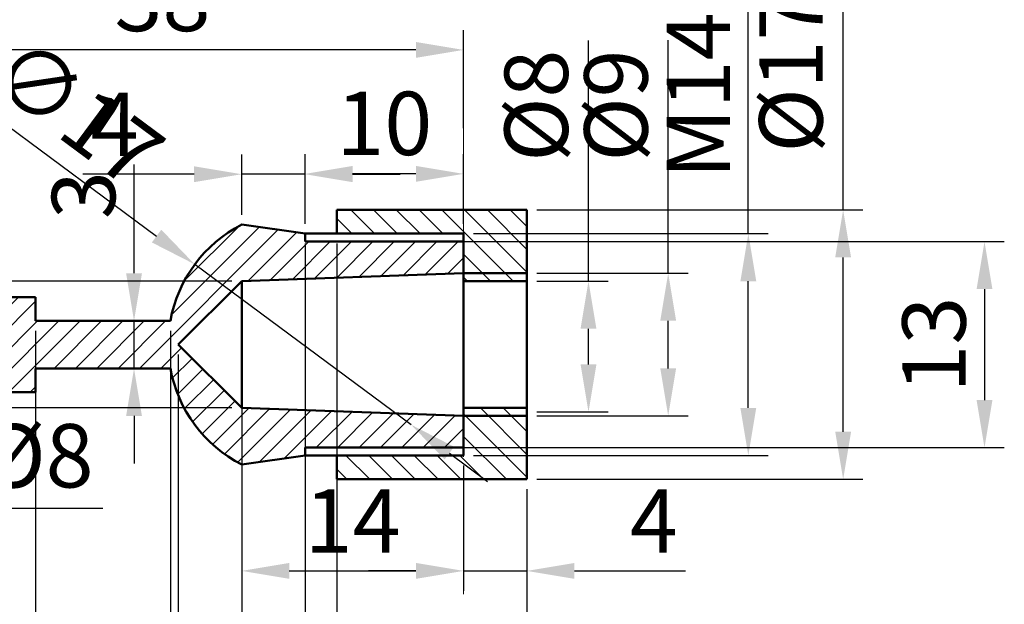
# Model space of a CAD drawing. Units: millimetres. Extents: x 139 to 291, y 28 to 164.
# Tile 3 of 5: x 174 to 236, y 81 to 118. Entities that reach past the tile are written whole.
import ezdxf

# ---------------------------------------------------------------- set-up
doc = ezdxf.new("R2010")
doc.units = ezdxf.units.MM
doc.linetypes.add('CENTER2', pattern=[28.575, 19.05, -3.175, 3.175, -3.175])
for name, color, linetype, lineweight in [('M-CNTR', 1, 'CENTER2', 18), ('M-DIMS', 2, 'Continuous', 25), ('M-HATC', 8, 'Continuous', 18), ('M-OUTL', 7, 'Continuous', 50)]:
    doc.layers.add(name, color=color, linetype=linetype, lineweight=lineweight)
doc.styles.get("Standard").update_dxf_attribs({"font": 'arial.ttf'})
doc.dimstyles.new('ISO-25', dxfattribs={"dimtxt": 4, "dimasz": 3, "dimexe": 1.25, "dimexo": 0.625, "dimtad": 1, "dimdec": 0, "dimtxsty": 'Standard', "dimcen": 2.5, "dimadec": 0, "dimazin": 0, "dimtfac": 1, "dimtdec": 0, "dimtmove": 0, "dimatfit": 3, "dimfxl": 1, "dimarcsym": 0})

# ---------------------------------------------------------------- blocks, each defined once
blk = doc.blocks.new('*D2')
at = {"layer": 'Defpoints', "color": 0, "transparency": 16777216}
for p in [(205.636, 101.663), (205.636, 93.413), (209.521, 93.413)]:
    blk.add_point(p, dxfattribs=at)
at = {"layer": 'M-DIMS', "color": 0, "lineweight": -2, "transparency": 16777216}
for p, q in [((209.521, 101.663), (209.521, 116.85)), ((206.261, 101.663), (210.771, 101.663)), ((209.521, 96.413), (209.521, 98.663)), ((206.261, 93.413), (210.771, 93.413))]:
    blk.add_line(p, q, dxfattribs=at)
at = {"layer": 'M-DIMS', "color": 0, "transparency": 16777216}
for points in [[(209.021, 98.663), (210.021, 98.663), (209.521, 101.663)], [(209.021, 96.413), (210.021, 96.413), (209.521, 93.413)]]:
    blk.add_solid(points, dxfattribs=at)
at = {"layer": 'M-DIMS', "color": 0, "transparency": 16777216, "insert": (206.742, 112.734), "char_height": 4, "attachment_point": 5, "rotation": 90}
blk.add_mtext('%%C8', dxfattribs=at)
blk = doc.blocks.new('*D3')
at = {"layer": 'Defpoints', "color": 0, "transparency": 16777216}
for p in [(205.636, 102.163), (205.636, 93.163), (214.551, 93.163)]:
    blk.add_point(p, dxfattribs=at)
at = {"layer": 'M-DIMS', "color": 0, "lineweight": -2, "transparency": 16777216}
for p, q in [((214.551, 102.163), (214.551, 116.863)), ((206.261, 102.163), (215.801, 102.163)), ((214.551, 96.163), (214.551, 99.163)), ((206.261, 93.163), (215.801, 93.163))]:
    blk.add_line(p, q, dxfattribs=at)
at = {"layer": 'M-DIMS', "color": 0, "transparency": 16777216}
for points in [[(214.051, 99.163), (215.051, 99.163), (214.551, 102.163)], [(214.051, 96.163), (215.051, 96.163), (214.551, 93.163)]]:
    blk.add_solid(points, dxfattribs=at)
at = {"layer": 'M-DIMS', "color": 0, "transparency": 16777216, "insert": (211.772, 112.747), "char_height": 4, "attachment_point": 5, "rotation": 90}
blk.add_mtext('%%C9', dxfattribs=at)
blk = doc.blocks.new('*D4')
at = {"layer": 'Defpoints', "color": 0, "transparency": 16777216}
for p in [(201.636, 104.663), (201.636, 90.663), (219.607, 90.663)]:
    blk.add_point(p, dxfattribs=at)
at = {"layer": 'M-DIMS', "color": 0, "lineweight": -2, "transparency": 16777216}
for p, q in [((219.607, 104.663), (219.607, 119.099)), ((202.261, 104.663), (220.857, 104.663)), ((219.607, 93.663), (219.607, 101.663)), ((202.261, 90.663), (220.857, 90.663))]:
    blk.add_line(p, q, dxfattribs=at)
at = {"layer": 'M-DIMS', "color": 0, "transparency": 16777216}
for points in [[(219.107, 101.663), (220.107, 101.663), (219.607, 104.663)], [(219.107, 93.663), (220.107, 93.663), (219.607, 90.663)]]:
    blk.add_solid(points, dxfattribs=at)
at = {"layer": 'M-DIMS', "color": 0, "transparency": 16777216, "insert": (216.974, 113.381), "char_height": 4, "attachment_point": 5, "rotation": 90}
blk.add_mtext('M14', dxfattribs=at)
blk = doc.blocks.new('*D5')
at = {"layer": 'Defpoints', "color": 0, "transparency": 16777216}
for p in [(205.636, 106.163), (205.636, 89.163), (225.591, 89.163)]:
    blk.add_point(p, dxfattribs=at)
at = {"layer": 'M-DIMS', "color": 0, "lineweight": -2, "transparency": 16777216}
for p, q in [((225.591, 106.163), (225.591, 120.495)), ((206.261, 106.163), (226.841, 106.163)), ((225.591, 92.163), (225.591, 103.163)), ((206.261, 89.163), (226.841, 89.163))]:
    blk.add_line(p, q, dxfattribs=at)
at = {"layer": 'M-DIMS', "color": 0, "transparency": 16777216}
for points in [[(225.091, 103.163), (226.091, 103.163), (225.591, 106.163)], [(225.091, 92.163), (226.091, 92.163), (225.591, 89.163)]]:
    blk.add_solid(points, dxfattribs=at)
at = {"layer": 'M-DIMS', "color": 0, "transparency": 16777216, "insert": (222.811, 114.829), "char_height": 4, "attachment_point": 5, "rotation": 90}
blk.add_mtext('%%C17', dxfattribs=at)
blk = doc.blocks.new('*D6')
at = {"layer": 'Defpoints', "color": 0, "transparency": 16777216}
for p in [(163.636, 116.256), (163.636, 110.703), (201.636, 110.703)]:
    blk.add_point(p, dxfattribs=at)
at = {"layer": 'M-DIMS', "color": 0, "lineweight": -2, "transparency": 16777216}
for p, q in [((163.636, 111.328), (163.636, 117.506)), ((201.636, 111.328), (201.636, 117.506)), ((198.636, 116.256), (166.636, 116.256))]:
    blk.add_line(p, q, dxfattribs=at)
at = {"layer": 'M-DIMS', "color": 0, "transparency": 16777216}
for points in [[(166.636, 116.756), (166.636, 115.756), (163.636, 116.256)], [(198.636, 116.756), (198.636, 115.756), (201.636, 116.256)]]:
    blk.add_solid(points, dxfattribs=at)
at = {"layer": 'M-DIMS', "color": 0, "transparency": 16777216, "insert": (182.636, 118.925), "char_height": 4, "attachment_point": 5}
blk.add_mtext('38', dxfattribs=at)
blk = doc.blocks.new('*D7')
at = {"layer": 'Defpoints', "color": 0, "transparency": 16777216}
for p in [(191.636, 108.435), (191.636, 104.663), (201.636, 104.663)]:
    blk.add_point(p, dxfattribs=at)
at = {"layer": 'M-DIMS', "color": 0, "lineweight": -2, "transparency": 16777216}
for p, q in [((191.636, 105.288), (191.636, 109.685)), ((201.636, 105.288), (201.636, 109.685)), ((198.636, 108.435), (194.636, 108.435))]:
    blk.add_line(p, q, dxfattribs=at)
at = {"layer": 'M-DIMS', "color": 0, "transparency": 16777216}
for points in [[(194.636, 108.935), (194.636, 107.935), (191.636, 108.435)], [(198.636, 108.935), (198.636, 107.935), (201.636, 108.435)]]:
    blk.add_solid(points, dxfattribs=at)
at = {"layer": 'M-DIMS', "color": 0, "transparency": 16777216, "insert": (196.636, 111.103), "char_height": 4, "attachment_point": 5}
blk.add_mtext('10', dxfattribs=at)
blk = doc.blocks.new('*D8')
at = {"layer": 'Defpoints', "color": 0, "transparency": 16777216}
for p in [(187.636, 108.413), (187.636, 105.232), (191.636, 104.663)]:
    blk.add_point(p, dxfattribs=at)
at = {"layer": 'M-DIMS', "color": 0, "lineweight": -2, "transparency": 16777216}
for p, q in [((187.636, 105.857), (187.636, 109.663)), ((191.636, 105.288), (191.636, 109.663)), ((184.636, 108.413), (177.619, 108.413)), ((191.636, 108.413), (187.636, 108.413)), ((194.636, 108.413), (197.636, 108.413))]:
    blk.add_line(p, q, dxfattribs=at)
at = {"layer": 'M-DIMS', "color": 0, "transparency": 16777216}
for points in [[(184.636, 108.913), (184.636, 107.913), (187.636, 108.413)], [(194.636, 108.913), (194.636, 107.913), (191.636, 108.413)]]:
    blk.add_solid(points, dxfattribs=at)
at = {"layer": 'M-DIMS', "color": 0, "transparency": 16777216, "insert": (179.627, 111.038), "char_height": 4, "attachment_point": 5}
blk.add_mtext('4', dxfattribs=at)
blk = doc.blocks.new('*D9')
at = {"layer": 'Defpoints', "color": 0, "transparency": 16777216}
for p in [(187.636, 93.663), (201.636, 90.663), (201.636, 83.384)]:
    blk.add_point(p, dxfattribs=at)
at = {"layer": 'M-DIMS', "color": 0, "lineweight": -2, "transparency": 16777216}
for p, q in [((187.636, 93.038), (187.636, 82.134)), ((201.636, 90.038), (201.636, 82.134)), ((190.636, 83.384), (198.636, 83.384))]:
    blk.add_line(p, q, dxfattribs=at)
at = {"layer": 'M-DIMS', "color": 0, "transparency": 16777216}
for points in [[(190.636, 83.884), (190.636, 82.884), (187.636, 83.384)], [(198.636, 83.884), (198.636, 82.884), (201.636, 83.384)]]:
    blk.add_solid(points, dxfattribs=at)
at = {"layer": 'M-DIMS', "color": 0, "transparency": 16777216, "insert": (194.636, 86.018), "char_height": 4, "attachment_point": 5}
blk.add_mtext('14', dxfattribs=at)
blk = doc.blocks.new('*D10')
at = {"layer": 'Defpoints', "color": 0, "transparency": 16777216}
for p in [(201.636, 89.163), (205.636, 89.163), (205.636, 83.381)]:
    blk.add_point(p, dxfattribs=at)
at = {"layer": 'M-DIMS', "color": 0, "lineweight": -2, "transparency": 16777216}
for p, q in [((201.636, 88.538), (201.636, 82.131)), ((205.636, 88.538), (205.636, 82.131)), ((198.636, 83.381), (195.636, 83.381)), ((201.636, 83.381), (205.636, 83.381)), ((208.636, 83.381), (215.653, 83.381))]:
    blk.add_line(p, q, dxfattribs=at)
at = {"layer": 'M-DIMS', "color": 0, "transparency": 16777216}
for points in [[(198.636, 83.881), (198.636, 82.881), (201.636, 83.381)], [(208.636, 83.881), (208.636, 82.881), (205.636, 83.381)]]:
    blk.add_solid(points, dxfattribs=at)
at = {"layer": 'M-DIMS', "color": 0, "transparency": 16777216, "insert": (213.644, 86.006), "char_height": 4, "attachment_point": 5}
blk.add_mtext('4', dxfattribs=at)
blk = doc.blocks.new('*D11')
at = {"layer": 'Defpoints', "color": 0, "transparency": 16777216}
for p in [(159.636, 94.663), (167.636, 94.663), (167.636, 87.351)]:
    blk.add_point(p, dxfattribs=at)
at = {"layer": 'M-DIMS', "color": 0, "lineweight": -2, "transparency": 16777216}
for p, q in [((159.636, 94.038), (159.636, 86.101)), ((167.636, 94.038), (167.636, 86.101)), ((162.636, 87.351), (164.636, 87.351)), ((167.636, 87.351), (178.868, 87.351))]:
    blk.add_line(p, q, dxfattribs=at)
at = {"layer": 'M-DIMS', "color": 0, "transparency": 16777216}
for points in [[(162.636, 87.851), (162.636, 86.851), (159.636, 87.351)], [(164.636, 87.851), (164.636, 86.851), (167.636, 87.351)]]:
    blk.add_solid(points, dxfattribs=at)
at = {"layer": 'M-DIMS', "color": 0, "transparency": 16777216, "insert": (174.752, 90.13), "char_height": 4, "attachment_point": 5}
blk.add_mtext('%%C8', dxfattribs=at)
blk = doc.blocks.new('*D12')
at = {"layer": 'Defpoints', "color": 0, "transparency": 16777216}
for p in [(180.338, 99.163), (180.338, 96.163), (180.843, 96.163)]:
    blk.add_point(p, dxfattribs=at)
at = {"layer": 'M-DIMS', "color": 0, "lineweight": -2, "transparency": 16777216}
for p, q in [((180.843, 102.163), (180.843, 109.033)), ((180.843, 96.163), (180.843, 99.163)), ((180.963, 99.163), (182.093, 99.163)), ((180.963, 96.163), (182.093, 96.163)), ((180.843, 93.163), (180.843, 90.163))]:
    blk.add_line(p, q, dxfattribs=at)
at = {"layer": 'M-DIMS', "color": 0, "transparency": 16777216}
for points in [[(180.343, 102.163), (181.343, 102.163), (180.843, 99.163)], [(180.343, 93.163), (181.343, 93.163), (180.843, 96.163)]]:
    blk.add_solid(points, dxfattribs=at)
at = {"layer": 'M-DIMS', "color": 0, "transparency": 16777216, "insert": (178.175, 107.098), "char_height": 4, "attachment_point": 5, "rotation": 90}
blk.add_mtext('3', dxfattribs=at)
blk = doc.blocks.new('*D36')
at = {"layer": 'Defpoints', "color": 0, "transparency": 16777216}
for p in [(152.636, 94.663), (205.636, 89.163), (205.636, 72.308)]:
    blk.add_point(p, dxfattribs=at)
at = {"layer": 'M-DIMS', "color": 0, "lineweight": -2, "transparency": 16777216}
for p, q in [((152.636, 94.038), (152.636, 71.058)), ((205.636, 88.538), (205.636, 71.058)), ((155.636, 72.308), (202.636, 72.308))]:
    blk.add_line(p, q, dxfattribs=at)
at = {"layer": 'M-DIMS', "color": 0, "transparency": 16777216}
for points in [[(155.636, 72.808), (155.636, 71.808), (152.636, 72.308)], [(202.636, 72.808), (202.636, 71.808), (205.636, 72.308)]]:
    blk.add_solid(points, dxfattribs=at)
at = {"layer": 'M-DIMS', "color": 0, "transparency": 16777216, "insert": (179.136, 74.977), "char_height": 4, "attachment_point": 5}
blk.add_mtext('53', dxfattribs=at)
blk = doc.blocks.new('*D37')
at = {"layer": 'Defpoints', "color": 0, "transparency": 16777216}
for p in [(174.636, 99.163), (183.137, 99.163), (183.137, 72.308)]:
    blk.add_point(p, dxfattribs=at)
at = {"layer": 'M-DIMS', "color": 0, "lineweight": -2, "transparency": 16777216}
for p, q in [((174.636, 98.538), (174.636, 71.058)), ((183.137, 98.538), (183.137, 71.058)), ((177.636, 72.308), (180.137, 72.308)), ((183.137, 72.308), (200.118, 72.308))]:
    blk.add_line(p, q, dxfattribs=at)
at = {"layer": 'M-DIMS', "color": 0, "transparency": 16777216}
for points in [[(177.636, 72.808), (177.636, 71.808), (174.636, 72.308)], [(180.137, 72.808), (180.137, 71.808), (183.137, 72.308)]]:
    blk.add_solid(points, dxfattribs=at)
at = {"layer": 'M-DIMS', "color": 0, "transparency": 16777216, "insert": (193.128, 74.976), "char_height": 4, "attachment_point": 5}
blk.add_mtext('8.501', dxfattribs=at)
blk = doc.blocks.new('*D38')
at = {"layer": 'Defpoints', "color": 0, "transparency": 16777216}
for p in [(187.636, 101.663), (183.636, 97.663), (187.636, 72.308)]:
    blk.add_point(p, dxfattribs=at)
at = {"layer": 'M-DIMS', "color": 0, "lineweight": -2, "transparency": 16777216}
for p, q in [((187.636, 101.038), (187.636, 71.058)), ((183.636, 97.038), (183.636, 71.058)), ((180.636, 72.308), (177.636, 72.308)), ((183.636, 72.308), (187.636, 72.308)), ((190.636, 72.308), (197.653, 72.308))]:
    blk.add_line(p, q, dxfattribs=at)
at = {"layer": 'M-DIMS', "color": 0, "transparency": 16777216}
for points in [[(180.636, 72.808), (180.636, 71.808), (183.636, 72.308)], [(190.636, 72.808), (190.636, 71.808), (187.636, 72.308)]]:
    blk.add_solid(points, dxfattribs=at)
at = {"layer": 'M-DIMS', "color": 0, "transparency": 16777216, "insert": (195.644, 74.933), "char_height": 4, "attachment_point": 5}
blk.add_mtext('4', dxfattribs=at)
blk = doc.blocks.new('*D39')
at = {"layer": 'Defpoints', "color": 0, "transparency": 16777216}
for p in [(187.636, 101.663), (144.186, 93.663), (187.636, 93.663)]:
    blk.add_point(p, dxfattribs=at)
at = {"layer": 'M-DIMS', "color": 0, "lineweight": -2, "transparency": 16777216}
for p, q in [((187.011, 101.663), (142.936, 101.663)), ((144.186, 98.663), (144.186, 96.663)), ((187.011, 93.663), (142.936, 93.663))]:
    blk.add_line(p, q, dxfattribs=at)
at = {"layer": 'M-DIMS', "color": 0, "transparency": 16777216}
for points in [[(143.686, 98.663), (144.686, 98.663), (144.186, 101.663)], [(143.686, 96.663), (144.686, 96.663), (144.186, 93.663)]]:
    blk.add_solid(points, dxfattribs=at)
at = {"layer": 'M-DIMS', "color": 0, "transparency": 16777216, "insert": (141.519, 97.663), "char_height": 4, "attachment_point": 5, "rotation": 90}
blk.add_mtext('8', dxfattribs=at)
blk = doc.blocks.new('*D40')
at = {"layer": 'Defpoints', "color": 0, "transparency": 16777216}
for p in [(191.636, 104.163), (191.636, 91.163), (234.511, 91.163)]:
    blk.add_point(p, dxfattribs=at)
at = {"layer": 'M-DIMS', "color": 0, "lineweight": -2, "transparency": 16777216}
for p, q in [((192.261, 104.163), (235.761, 104.163)), ((234.511, 101.163), (234.511, 94.163)), ((192.261, 91.163), (235.761, 91.163))]:
    blk.add_line(p, q, dxfattribs=at)
at = {"layer": 'M-DIMS', "color": 0, "transparency": 16777216}
for points in [[(234.011, 101.163), (235.011, 101.163), (234.511, 104.163)], [(234.011, 94.163), (235.011, 94.163), (234.511, 91.163)]]:
    blk.add_solid(points, dxfattribs=at)
at = {"layer": 'M-DIMS', "color": 0, "transparency": 16777216, "insert": (231.842, 97.663), "char_height": 4, "attachment_point": 5, "rotation": 90}
blk.add_mtext('13', dxfattribs=at)
blk = doc.blocks.new('*D41')
at = {"layer": 'Defpoints', "color": 0, "transparency": 16777216}
for p in [(191.636, 104.663), (193.636, 104.663), (193.636, 72.308)]:
    blk.add_point(p, dxfattribs=at)
at = {"layer": 'M-DIMS', "color": 0, "lineweight": -2, "transparency": 16777216}
for p, q in [((191.636, 104.038), (191.636, 71.058)), ((193.636, 104.038), (193.636, 71.058)), ((188.636, 72.308), (185.636, 72.308)), ((191.636, 72.308), (193.636, 72.308)), ((196.636, 72.308), (203.535, 72.308))]:
    blk.add_line(p, q, dxfattribs=at)
at = {"layer": 'M-DIMS', "color": 0, "transparency": 16777216}
for points in [[(188.636, 72.808), (188.636, 71.808), (191.636, 72.308)], [(196.636, 72.808), (196.636, 71.808), (193.636, 72.308)]]:
    blk.add_solid(points, dxfattribs=at)
at = {"layer": 'M-DIMS', "color": 0, "transparency": 16777216, "insert": (201.586, 74.942), "char_height": 4, "attachment_point": 5}
blk.add_mtext('2', dxfattribs=at)
blk = doc.blocks.new('*D57')
at = {"layer": 'Defpoints', "color": 0, "transparency": 16777216}
for p in [(184.675, 102.725), (198.332, 92.602)]:
    blk.add_point(p, dxfattribs=at)
at = {"layer": 'M-DIMS', "color": 0, "lineweight": -2, "transparency": 16777216}
for p, q in [((170.751, 113.046), (182.265, 104.511)), ((198.332, 92.602), (184.675, 102.725)), ((200.743, 90.815), (203.153, 89.029))]:
    blk.add_line(p, q, dxfattribs=at)
at = {"layer": 'M-DIMS', "color": 0, "transparency": 16777216}
for points in [[(182.563, 104.913), (181.967, 104.11), (184.675, 102.725)], [(201.04, 91.217), (200.445, 90.414), (198.332, 92.602)]]:
    blk.add_solid(points, dxfattribs=at)
at = {"layer": 'M-DIMS', "color": 0, "transparency": 16777216, "insert": (176.958, 111.904), "char_height": 4, "attachment_point": 5, "rotation": 323.45299}
blk.add_mtext('∅17', dxfattribs=at)

msp = doc.modelspace()

# ---------------------------------------------------------------- hatches: boundary and pattern name
at = {"layer": 'M-HATC'}
h = msp.add_hatch(dxfattribs=at)
h.set_pattern_fill('ANSI31', color=256, scale=0.32, angle=90)
h.set_pattern_definition([(135, (0, -8.2379), (-0.7184205, -0.7184205), [])])
h.paths.add_polyline_path([(205.6359, 106.1632), (193.6359, 106.1632), (193.6359, 104.6632), (201.6359, 104.6632), (201.6359, 102.1632), (205.6359, 102.1632)])
h.paths.add_polyline_path([(205.6359, 102.1632), (201.6359, 102.1632), (201.6359, 101.6632), (205.6359, 101.6632)])
h.paths.add_polyline_path([(205.6359, 93.1632), (201.6359, 93.1632), (201.6359, 90.6632), (193.6359, 90.6632), (193.6359, 89.1632), (205.6359, 89.1632)])
h.paths.add_polyline_path([(205.6359, 93.6632), (201.6359, 93.6632), (201.6359, 93.1632), (205.6359, 93.1632)])
h = msp.add_hatch(dxfattribs=at)
h.set_pattern_fill('ANSI31', color=256, scale=0.3)
h.set_pattern_definition([(45, (0, -8.2379), (-0.6735192, 0.6735192), [])])
h.paths.add_polyline_path([(174.6359, 99.1632), (174.6359, 100.6632), (167.6359, 100.6632), (167.6359, 94.6632), (174.6359, 94.6632), (174.6359, 96.1632), (183.1373, 96.1632, 0.2343961), (187.6359, 90.0943), (191.6359, 90.6632), (191.6359, 91.1632), (201.6359, 91.1632), (201.6359, 93.1632), (187.6359, 93.6632), (183.6359, 97.6632), (187.6359, 101.6632), (201.6359, 102.1632), (201.6359, 104.1632), (191.6359, 104.1632), (191.6359, 104.6632), (187.6359, 105.2322, 0.2343961), (183.1373, 99.1632)])
h.paths.add_polyline_path([(159.6359, 94.6632), (159.6359, 100.6632), (152.6359, 100.6632), (152.6359, 94.6632)])

# ---------------------------------------------------------------- linework, layer by layer
at = {"layer": 'M-CNTR'}
msp.add_line((201.6359, 115.9753), (201.6359, 81.9185), dxfattribs=at)
at = {"layer": 'M-OUTL'}
for p, q in [((193.6359, 106.1632), (205.6359, 106.1632)), ((193.6359, 104.6632), (193.6359, 106.1632)), ((205.6359, 97.6632), (205.6359, 106.1632)), ((191.6359, 104.6632), (187.6359, 105.2322)), ((201.6359, 104.6632), (191.6359, 104.6632)), ((191.6359, 104.6632), (191.6359, 104.1632)), ((201.6359, 102.1632), (201.6359, 104.6632)), ((191.6359, 104.1632), (201.6359, 104.1632)), ((187.6359, 101.6632), (201.6359, 102.1632)), ((201.6359, 101.6632), (201.6359, 102.1632)), ((201.6359, 102.1632), (205.6359, 102.1632)), ((187.6359, 101.6632), (183.6359, 97.6632)), ((187.6359, 97.6632), (187.6359, 101.6632)), ((201.6359, 101.6632), (205.6359, 101.6632)), ((201.6359, 101.6632), (201.6359, 93.6632)), ((163.6359, 100.6632), (174.6359, 100.6632)), ((174.6359, 100.6632), (174.6359, 99.1632)), ((183.1373, 99.1632), (174.6359, 99.1632)), ((187.6359, 93.6632), (183.6359, 97.6632)), ((187.6359, 97.6632), (187.6359, 93.6632)), ((205.6359, 97.6632), (205.6359, 89.1632)), ((183.1373, 96.1632), (174.6359, 96.1632)), ((174.6359, 96.1632), (174.6359, 94.6632)), ((174.6359, 94.6632), (152.6359, 94.6632)), ((187.6359, 93.6632), (201.6359, 93.1632)), ((201.6359, 93.6632), (205.6359, 93.6632)), ((201.6359, 93.1632), (201.6359, 93.6632)), ((201.6359, 93.1632), (201.6359, 90.6632)), ((201.6359, 93.1632), (205.6359, 93.1632)), ((191.6359, 90.6632), (191.6359, 91.1632)), ((191.6359, 91.1632), (201.6359, 91.1632)), ((191.6359, 90.6632), (187.6359, 90.0943)), ((201.6359, 90.6632), (191.6359, 90.6632)), ((193.6359, 89.1632), (193.6359, 90.6632)), ((205.6359, 89.1632), (193.6359, 89.1632))]:
    msp.add_line(p, q, dxfattribs=at)
for start, end in [(117.068734, 169.835751), (190.164249, 242.931266)]:
    msp.add_arc((191.5039, 97.6632), 8.5, start, end, dxfattribs=at)

# ---------------------------------------------------------------- dimensions: what is measured, and where the dimension line sits
at = {"layer": 'M-DIMS'}
for base, p1, p2, override, picture, middle in [((163.6359, 116.2564), (201.6359, 110.7027), (163.6359, 110.7027), {"dimclrd": 0, "dimclre": 0, "dimclrt": 0}, '*D6', (182.6359, 118.9251)), ((191.6359, 108.4353), (201.6359, 104.6632), (191.6359, 104.6632), {"dimclrd": 0, "dimclre": 0, "dimclrt": 0}, '*D7', (196.6359, 111.1026)), ((187.6359, 108.4132), (191.6359, 104.6632), (187.6359, 105.2322), {"dimclrd": 0, "dimclre": 0, "dimclrt": 0}, '*D8', (179.6275, 111.0382)), ((193.6359, 72.3085), (191.6359, 104.6632), (193.6359, 104.6632), {"dimdec": 0, "dimlfac": 1, "dimrnd": 0, "dimzin": 0, "dimdsep": 46, "dimlunit": 2}, '*D41', (201.5855, 74.9417)), ((187.6359, 72.3085), (183.6359, 97.6632), (187.6359, 101.6632), {"dimdec": 0, "dimlfac": 1, "dimrnd": 0, "dimzin": 0, "dimdsep": 46, "dimlunit": 2}, '*D38', (195.6442, 74.9335)), ((183.1373, 72.3085), (174.6359, 99.1632), (183.1373, 99.1632), {"dimdec": 3, "dimlfac": 1, "dimrnd": 0, "dimzin": 0, "dimdsep": 46, "dimlunit": 2}, '*D37', (193.1279, 74.9758)), ((205.6359, 72.3085), (152.6359, 94.6632), (205.6359, 89.1632), {"dimdec": 0, "dimlfac": 1, "dimrnd": 0, "dimzin": 0, "dimdsep": 46, "dimlunit": 2}, '*D36', (179.1359, 74.9771)), ((201.6359, 83.3844), (187.6359, 93.6632), (201.6359, 90.6632), {"dimclrd": 0, "dimclre": 0, "dimclrt": 0}, '*D9', (194.6359, 86.0176)), ((205.6359, 83.3807), (201.6359, 89.1632), (205.6359, 89.1632), {"dimclrd": 0, "dimclre": 0, "dimclrt": 0}, '*D10', (213.6442, 86.0057))]:
    dim = msp.add_linear_dim(base=base, p1=p1, p2=p2, dimstyle='ISO-25', override=override, dxfattribs=at)
    dim.commit()
    dim.dimension.update_dxf_attribs({"geometry": picture, "text_midpoint": middle})
for base, p1, p2, text, picture, middle in [((225.5906, 89.1632), (205.6359, 106.1632), (205.6359, 89.1632), '%%C<>', '*D5', (225.5906, 114.8292)), ((219.6067, 90.6632), (201.6359, 104.6632), (201.6359, 90.6632), 'M<>', '*D4', (219.6067, 113.381)), ((209.521, 93.4132), (205.6359, 101.6632), (205.6359, 93.4132), '%%C<>', '*D2', (209.521, 112.7336)), ((214.551, 93.1632), (205.6359, 102.1632), (205.6359, 93.1632), '%%C<>', '*D3', (214.551, 112.7473))]:
    dim = msp.add_linear_dim(base=base, p1=p1, p2=p2, angle=90, text=text, dimstyle='ISO-25', override={"dimclrd": 0, "dimclre": 0, "dimclrt": 0}, dxfattribs=at)
    dim.commit()
    dim.dimension.update_dxf_attribs({"geometry": picture, "text_midpoint": middle, "dimtype": 160})
dim = msp.add_diameter_dim_2p(p1=(198.3325, 92.6016), p2=(184.6752, 102.7248), dimstyle='ISO-25', override={"dimdec": 0, "dimlfac": 1, "dimrnd": 0, "dimzin": 0, "dimdsep": 46, "dimlunit": 2}, dxfattribs=at)
dim.commit()
dim.dimension.update_dxf_attribs({"geometry": '*D57', "text_midpoint": (175.3032, 109.6717), "dimtype": 163})
dim = msp.add_linear_dim(base=(180.8434, 96.1632), p1=(180.3385, 99.1632), p2=(180.3385, 96.1632), angle=90, dimstyle='ISO-25', override={"dimclrd": 0, "dimclre": 0, "dimclrt": 0}, dxfattribs=at)
dim.commit()
dim.dimension.update_dxf_attribs({"geometry": '*D12', "text_midpoint": (180.8434, 107.0979), "dimtype": 160})
for base, p1, p2, picture, middle in [((234.5106, 91.1632), (191.6359, 104.1632), (191.6359, 91.1632), '*D40', (231.8419, 97.6632)), ((144.1859, 93.6632), (187.6359, 101.6632), (187.6359, 93.6632), '*D39', (141.5186, 97.6632))]:
    dim = msp.add_linear_dim(base=base, p1=p1, p2=p2, angle=90, dimstyle='ISO-25', override={"dimdec": 0, "dimlfac": 1, "dimrnd": 0, "dimzin": 0, "dimdsep": 46, "dimlunit": 2}, dxfattribs=at)
    dim.commit()
    dim.dimension.update_dxf_attribs({"geometry": picture, "text_midpoint": middle})
dim = msp.add_linear_dim(base=(167.6359, 87.3506), p1=(159.6359, 94.6632), p2=(167.6359, 94.6632), text='%%C<>', dimstyle='ISO-25', override={"dimclrd": 0, "dimclre": 0, "dimclrt": 0}, dxfattribs=at)
dim.commit()
dim.dimension.update_dxf_attribs({"geometry": '*D11', "text_midpoint": (174.752, 90.1297)})

doc.saveas('drawing.dxf')
